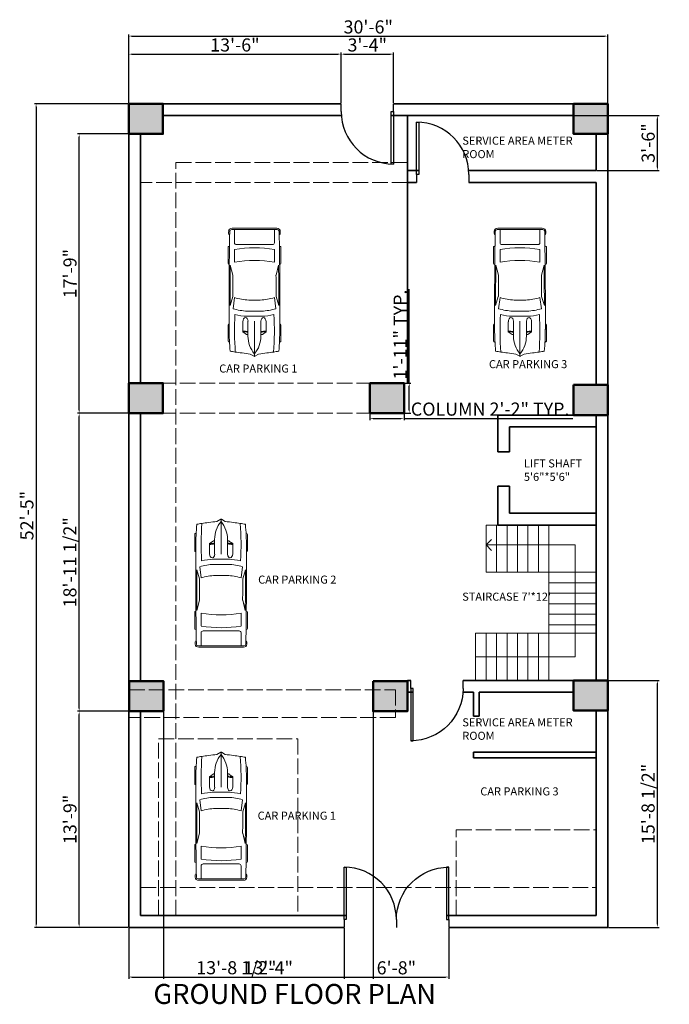
# Model space of a CAD drawing. Units: inches. Extents: x 1964 to 3462, y 1879 to 2909.
# Tile 1 of 4: x 1964 to 2460, y 2008 to 2759. Entities that reach past the tile are written whole.
import ezdxf

# ---------------------------------------------------------------- set-up
doc = ezdxf.new("R2010")
doc.units = ezdxf.units.IN
doc.linetypes.add('ACAD_ISO02W100', pattern=[15, 12, -3])
for name, color, linetype, lineweight in [('A-ANNO-DIMS', 2, 'Continuous', 18), ('A-ANNO-TEXT', 7, 'Continuous', 35), ('A-AREA-IDEN', 7, 'Continuous', 18), ('A-COLS', 1, 'Continuous', 50), ('A-COLS-PATT', 252, 'Continuous', 13), ('A-DOOR', 4, 'Continuous', 25), ('A-EQPM-VEHI', 8, 'Continuous', 13), ('A-FLOR-EVTR', 7, 'Continuous', 35), ('A-FLOR-OVHD', 8, 'ACAD_ISO02W100', 18), ('A-FLOR-PARK', 8, 'ACAD_ISO02W100', 18), ('A-FLOR-STRS', 3, 'Continuous', 18), ('A-WALL', 7, 'Continuous', 35)]:
    doc.layers.add(name, color=color, linetype=linetype, lineweight=lineweight)
doc.styles.get("Standard").update_dxf_attribs({"font": 'arial.ttf'})
doc.dimstyles.new('ISO-25', dxfattribs={"dimtxt": 10, "dimasz": 2.5, "dimexe": 1.25, "dimexo": 0.625, "dimtad": 1, "dimdec": 0, "dimlunit": 4, "dimtxsty": 'Standard', "dimcen": 2.5, "dimadec": 0, "dimazin": 0, "dimtfac": 1, "dimtdec": 0, "dimtmove": 0, "dimatfit": 3, "dimfxl": 1, "dimarcsym": 0})

# ---------------------------------------------------------------- blocks, each defined once
blk = doc.blocks.new('*U2')
for p, q in [((0, 0), (0, -6)), ((40, 0), (40, -6))]:
    blk.add_line(p, q)
blk.add_lwpolyline([(0, 0), (0, 40), (1.75, 40), (1.75, 0)], close=True)
blk.add_arc((0, 0), 40, 0, 90)
blk = doc.blocks.new('*U5')
for p, q in [((21.1, 37.4), (21.1, 36.8)), ((46.6, 38.9), (22.4, 38.9)), ((47.8, 37.4), (47.8, 37.4)), ((70, 31.5), (86.4, 29.4)), ((88, 31.9), (74.8, 35.9)), ((134.3, 35.6), (119.3, 31.8)), ((135.5, 37.1), (135.5, 37.4)), ((136.7, 38.9), (160.9, 38.9)), ((138.4, 29.4), (157.2, 29.4)), ((162.1, 37.4), (162.1, 36.8)), ((186.5, 29.4), (167, 29.4)), ((186.5, -33.5), (186.5, 33.5)), ((188.4, -32.8), (188.4, 32.8)), ((32.3, 11.6), (36.1, 17.2)), ((36.1, 17.2), (50.9, 17.2)), ((164.5, 26.4), (164.5, -26.4)), ((3.3, 6.1), (0.1, 0.4)), ((29.8, 9.5), (51.7, 9.5)), ((32.1, 9.5), (32.1, 11.2)), ((58.9, -10.8), (58.9, 10.8)), ((66.6, -10.5), (66.6, 10.5)), ((82.7, 8.5), (82.7, -8.5)), ((186.5, -10.5), (186.5, 10.5)), ((0, 0), (51.7, 0)), ((0.1, -0.4), (3.3, -6.1)), ((29.8, -9.5), (51.7, -9.5)), ((32.1, -9.5), (32.1, -11.2)), ((32.3, -11.6), (36.1, -17.2)), ((36.1, -17.2), (50.9, -17.2)), ((21.1, -37.4), (21.1, -36.8)), ((46.6, -38.9), (22.4, -38.9)), ((47.8, -37.4), (47.8, -37.4)), ((86.4, -29.4), (70, -31.5)), ((88, -31.9), (74.8, -35.9)), ((134.3, -35.6), (119.3, -31.8)), ((135.5, -37.1), (135.5, -37.4)), ((136.7, -38.9), (160.9, -38.9)), ((157.2, -29.4), (138.4, -29.4)), ((162.1, -37.4), (162.1, -36.8)), ((167, -29.4), (186.5, -29.4))]:
    blk.add_line(p, q)
for centre, major_axis, ratio, start_param, end_param in [((266, -27.5), (0, 313.3), 0.842304, 1.367076, 1.39176), ((37.5, -594), (0, -623.3), 0.842304, 3.096046, 3.200911), ((41.2, -490.9), (0, 528.2), 0.842304, 0.00281, 0.075598), ((22.4, 37.4), (0, -1.48), 0.842304, 3.141593, 4.712389), ((64.5, -10555.6), (0, 10593), 0.842304, -0.013397, 0.002797), ((46.6, 37.4), (0, 1.48), 0.842304, -1.570796, 0), ((135.3, 5.4), (0, 81.8), 0.842304, 1.245306, 1.50788), ((64.5, -10555.6), (0, -10591.5), 0.842304, 3.133765, 3.140441), ((149.6, 2.8), (0, -79.6), 0.842304, 4.372215, 4.640744), ((95.8, -3666.4), (0, -3698.2), 0.842304, 3.134049, 3.144098), ((136.7, 37.4), (0, -1.48), 0.842304, 3.141593, 4.712389), ((17.1, 0), (0, 147), 0.842304, 4.511394, 4.913384), ((35.9, 0), (0, 147), 0.842304, 4.511394, 4.913384), ((160.9, 37.4), (0, 1.48), 0.842304, -1.570796, 0), ((167, 26.4), (0, 2.96), 0.842304, 0, 1.570796), ((180.6, 35.8), (0, 2.22), 0.842304, -0.013017, 1.249894), ((64.5, -10556.4), (0, 10595.3), 0.842304, -0.013397, -0.013017), ((184, 32.8), (0, -5.25), 0.842304, 1.570796, 3.128196), ((184, 33.5), (0, -2.96), 0.842304, 1.570796, 3.128196), ((-204.5, 52.4), (0, -251), 0.842304, 1.385369, 1.434372), ((259.2, -27.5), (0, -305.3), 0.842304, 4.528606, 4.561838), ((13, 17), (0, 27.4), 0.842304, 4.435146, 4.718221), ((14.2, 17), (0, 27.4), 0.842304, 4.435146, 4.718221), ((50.8, 13.3), (6.34, -0.36), 0.603834, -1.395552, 1.581315), ((134.4, 5.4), (0, -89.8), 0.842304, 4.449482, 4.652344), ((0.6, 0), (0, -0.74), 0.842304, 4.131459, 5.293319), ((29.8, -46.7), (0, 56.2), 0.842304, 0, 0.590319), ((32.7, 11.2), (0, 0.74), 0.842304, 0.879714, 1.570796), ((-204.5, -52.4), (0, 251), 0.842304, -1.434372, -1.385369), ((29.8, 46.7), (0, 56.2), 0.842304, 2.551274, 3.141593), ((32.7, -11.2), (0, -0.74), 0.842304, 4.712389, 5.403472), ((13, -17), (0, -27.4), 0.842304, 1.564964, 1.848039), ((14.2, -17), (0, -27.4), 0.842304, 1.564964, 1.848039), ((134.4, -5.4), (0, -89.8), 0.842304, -1.510751, -1.307889), ((135.3, -5.4), (0, -81.8), 0.842304, -1.50788, -1.245306), ((149.6, -2.8), (0, -79.6), 0.842304, -1.499151, -1.230623), ((259.2, 27.5), (0, 305.3), 0.842304, 1.721348, 1.754579), ((266, 27.5), (0, 313.3), 0.842304, 1.749832, 1.774517), ((37.5, 594), (0, -623.3), 0.842304, -0.059319, 0.045547), ((167, -26.4), (0, -2.96), 0.842304, 4.712389, 6.283185), ((41.2, 490.9), (0, -528.2), 0.842304, -0.075598, -0.00281), ((22.4, -37.4), (0, 1.48), 0.842304, 1.570796, 3.141593), ((64.5, 10555.6), (0, 10593), 0.842304, 3.138796, 3.15499), ((46.6, -37.4), (0, -1.48), 0.842304, 0, 1.570796), ((64.5, 10555.6), (0, -10591.5), 0.842304, 0.001152, 0.007828), ((95.8, 3666.4), (0, -3698.2), 0.842304, -0.002505, 0.007544), ((136.7, -37.4), (0, -1.48), 0.842304, -1.570796, 0), ((160.9, -37.4), (0, 1.48), 0.842304, 3.141593, 4.712389), ((180.6, -35.8), (0, -2.22), 0.842304, -1.249894, 0.013017), ((64.5, 10556.4), (0, 10595.3), 0.842304, 3.15461, 3.15499), ((184, -32.8), (0, -5.25), 0.842304, 0.013397, 1.570796), ((184, -33.5), (0, 2.96), 0.842304, 3.15499, 4.712389)]:
    blk.add_ellipse(centre, major_axis=major_axis, ratio=ratio, start_param=start_param, end_param=end_param)
at = {"extrusion": (0, 0, -1)}
blk.add_ellipse((50.8, -13.3), major_axis=(6.34, 0.36), ratio=0.603834, start_param=-1.395552, end_param=1.581315, dxfattribs=at)
blk = doc.blocks.new('*D7')
at = {"layer": 'A-ANNO-DIMS', "color": 0, "lineweight": -2, "transparency": 16777216}
for p, q in [((2047.23, 2695.8), (2047.23, 2748.04)), ((2049.73, 2746.79), (2410.73, 2746.79)), ((2413.23, 2695.8), (2413.23, 2748.04))]:
    blk.add_line(p, q, dxfattribs=at)
at = {"layer": 'A-ANNO-DIMS', "color": 0, "lineweight": 100, "transparency": 16777216}
for points in [[(2049.73, 2747.21), (2049.73, 2746.37), (2047.23, 2746.79)], [(2410.73, 2747.21), (2410.73, 2746.37), (2413.23, 2746.79)]]:
    blk.add_solid(points, dxfattribs=at)
at = {"layer": 'Defpoints', "color": 0, "lineweight": 100, "transparency": 16777216}
for p in [(2413.23, 2746.79), (2047.23, 2695.18), (2413.23, 2695.18)]:
    blk.add_point(p, dxfattribs=at)
at = {"layer": 'A-ANNO-DIMS', "color": 0, "transparency": 16777216, "insert": (2230.23, 2752.52), "char_height": 10, "attachment_point": 5}
blk.add_mtext('30\'-6"', dxfattribs=at)
blk = doc.blocks.new('*D8')
at = {"layer": 'A-ANNO-DIMS', "color": 0, "lineweight": -2, "transparency": 16777216}
for p, q in [((2046.6, 2695.18), (1975.23, 2695.18)), ((1976.48, 2692.68), (1976.48, 2068.92)), ((2046.6, 2066.42), (1975.23, 2066.42))]:
    blk.add_line(p, q, dxfattribs=at)
at = {"layer": 'A-ANNO-DIMS', "color": 0, "lineweight": 100, "transparency": 16777216}
for points in [[(1976.07, 2692.68), (1976.9, 2692.68), (1976.48, 2695.18)], [(1976.07, 2068.92), (1976.9, 2068.92), (1976.48, 2066.42)]]:
    blk.add_solid(points, dxfattribs=at)
at = {"layer": 'Defpoints', "color": 0, "lineweight": 100, "transparency": 16777216}
for p in [(2047.23, 2695.18), (1976.48, 2066.42), (2047.23, 2066.42)]:
    blk.add_point(p, dxfattribs=at)
at = {"layer": 'A-ANNO-DIMS', "color": 0, "transparency": 16777216, "insert": (1970.75, 2380.8), "char_height": 10, "attachment_point": 5, "rotation": 90}
blk.add_mtext('52\'-5"', dxfattribs=at)
blk = doc.blocks.new('COL-RECT-26x23')
blk.add_lwpolyline([(0, 23.08), (26.15, 23.08), (26.15, 0), (0, 0)], close=True)
blk = doc.blocks.new('*D23')
at = {"layer": 'A-ANNO-DIMS', "color": 0, "lineweight": -2, "transparency": 16777216}
for p, q in [((2231.42, 2458.3), (2231.42, 2453.75)), ((2257.57, 2458.3), (2257.57, 2453.75)), ((2233.92, 2455), (2255.07, 2455)), ((2257.57, 2455), (2386.58, 2455))]:
    blk.add_line(p, q, dxfattribs=at)
at = {"layer": 'A-ANNO-DIMS', "color": 0, "lineweight": 100, "transparency": 16777216}
for points in [[(2233.92, 2455.42), (2233.92, 2454.59), (2231.42, 2455)], [(2255.07, 2455.42), (2255.07, 2454.59), (2257.57, 2455)]]:
    blk.add_solid(points, dxfattribs=at)
at = {"layer": 'Defpoints', "color": 0, "lineweight": 100, "transparency": 16777216}
for p in [(2231.42, 2458.93), (2257.57, 2458.93), (2257.57, 2455)]:
    blk.add_point(p, dxfattribs=at)
at = {"layer": 'A-ANNO-DIMS', "color": 0, "transparency": 16777216, "insert": (2323.32, 2460.8), "char_height": 10, "attachment_point": 5}
blk.add_mtext('COLUMN 2\'-2" TYP.', dxfattribs=at)
blk = doc.blocks.new('*D24')
at = {"layer": 'A-ANNO-DIMS', "color": 0, "lineweight": -2, "transparency": 16777216}
for p, q in [((2261.49, 2482.01), (2261.49, 2553.54)), ((2258.19, 2482.01), (2262.74, 2482.01)), ((2261.49, 2461.43), (2261.49, 2479.51)), ((2258.19, 2458.93), (2262.74, 2458.93))]:
    blk.add_line(p, q, dxfattribs=at)
at = {"layer": 'A-ANNO-DIMS', "color": 0, "lineweight": 100, "transparency": 16777216}
for points in [[(2261.08, 2479.51), (2261.91, 2479.51), (2261.49, 2482.01)], [(2261.08, 2461.43), (2261.91, 2461.43), (2261.49, 2458.93)]]:
    blk.add_solid(points, dxfattribs=at)
at = {"layer": 'Defpoints', "color": 0, "lineweight": 100, "transparency": 16777216}
for p in [(2257.57, 2482.01), (2261.49, 2482.01), (2257.57, 2458.93)]:
    blk.add_point(p, dxfattribs=at)
at = {"layer": 'A-ANNO-DIMS', "color": 0, "transparency": 16777216, "insert": (2255.84, 2519.03), "char_height": 10, "attachment_point": 5, "rotation": 90}
blk.add_mtext('1\'-11" TYP.', dxfattribs=at)
blk = doc.blocks.new('*D43')
at = {"layer": 'A-ANNO-DIMS', "color": 0, "lineweight": -2, "transparency": 16777216}
for p, q in [((2047.23, 2065.79), (2047.23, 2027.32)), ((2211.69, 2065.79), (2211.69, 2027.32)), ((2049.73, 2028.57), (2209.19, 2028.57))]:
    blk.add_line(p, q, dxfattribs=at)
at = {"layer": 'A-ANNO-DIMS', "color": 0, "lineweight": 100, "transparency": 16777216}
for points in [[(2049.73, 2028.98), (2049.73, 2028.15), (2047.23, 2028.57)], [(2209.19, 2028.98), (2209.19, 2028.15), (2211.69, 2028.57)]]:
    blk.add_solid(points, dxfattribs=at)
at = {"layer": 'Defpoints', "color": 0, "lineweight": 100, "transparency": 16777216}
for p in [(2047.23, 2066.42), (2211.69, 2066.42), (2211.69, 2028.57)]:
    blk.add_point(p, dxfattribs=at)
at = {"layer": 'A-ANNO-DIMS', "color": 0, "transparency": 16777216, "insert": (2129.46, 2034.37), "char_height": 10, "attachment_point": 5}
blk.add_mtext('13\'-8 1/2"', dxfattribs=at)
blk = doc.blocks.new('*D44')
at = {"layer": 'A-ANNO-DIMS', "color": 0, "lineweight": -2, "transparency": 16777216}
for p, q in [((2211.69, 2065.79), (2211.69, 2027.32)), ((2291.69, 2065.79), (2291.69, 2027.32)), ((2214.19, 2028.57), (2289.19, 2028.57))]:
    blk.add_line(p, q, dxfattribs=at)
at = {"layer": 'A-ANNO-DIMS', "color": 0, "lineweight": 100, "transparency": 16777216}
for points in [[(2214.19, 2028.98), (2214.19, 2028.15), (2211.69, 2028.57)], [(2289.19, 2028.98), (2289.19, 2028.15), (2291.69, 2028.57)]]:
    blk.add_solid(points, dxfattribs=at)
at = {"layer": 'Defpoints', "color": 0, "lineweight": 100, "transparency": 16777216}
for p in [(2211.69, 2066.42), (2291.69, 2066.42), (2291.69, 2028.57)]:
    blk.add_point(p, dxfattribs=at)
at = {"layer": 'A-ANNO-DIMS', "color": 0, "transparency": 16777216, "insert": (2251.69, 2034.3), "char_height": 10, "attachment_point": 5}
blk.add_mtext('6\'-8"', dxfattribs=at)
blk = doc.blocks.new('*D45')
at = {"layer": 'A-ANNO-DIMS', "color": 0, "lineweight": -2, "transparency": 16777216}
for p, q in [((2046.96, 2231.42), (2008.13, 2231.42)), ((2009.38, 2068.92), (2009.38, 2228.92)), ((2046.6, 2066.42), (2008.13, 2066.42))]:
    blk.add_line(p, q, dxfattribs=at)
at = {"layer": 'A-ANNO-DIMS', "color": 0, "lineweight": 100, "transparency": 16777216}
for points in [[(2008.96, 2228.92), (2009.8, 2228.92), (2009.38, 2231.42)], [(2008.96, 2068.92), (2009.8, 2068.92), (2009.38, 2066.42)]]:
    blk.add_solid(points, dxfattribs=at)
at = {"layer": 'Defpoints', "color": 0, "lineweight": 100, "transparency": 16777216}
for p in [(2009.38, 2231.42), (2047.58, 2231.42), (2047.23, 2066.42)]:
    blk.add_point(p, dxfattribs=at)
at = {"layer": 'A-ANNO-DIMS', "color": 0, "transparency": 16777216, "insert": (2003.64, 2148.92), "char_height": 10, "attachment_point": 5, "rotation": 90}
blk.add_mtext('13\'-9"', dxfattribs=at)
blk = doc.blocks.new('*D46')
at = {"layer": 'A-ANNO-DIMS', "color": 0, "lineweight": -2, "transparency": 16777216}
for p, q in [((2046.6, 2458.93), (2008.13, 2458.93)), ((2009.38, 2233.92), (2009.38, 2456.43)), ((2046.96, 2231.42), (2008.13, 2231.42))]:
    blk.add_line(p, q, dxfattribs=at)
at = {"layer": 'A-ANNO-DIMS', "color": 0, "lineweight": 100, "transparency": 16777216}
for points in [[(2008.96, 2456.43), (2009.8, 2456.43), (2009.38, 2458.93)], [(2008.96, 2233.92), (2009.8, 2233.92), (2009.38, 2231.42)]]:
    blk.add_solid(points, dxfattribs=at)
at = {"layer": 'Defpoints', "color": 0, "lineweight": 100, "transparency": 16777216}
for p in [(2009.38, 2458.93), (2047.23, 2458.93), (2047.58, 2231.42)]:
    blk.add_point(p, dxfattribs=at)
at = {"layer": 'A-ANNO-DIMS', "color": 0, "transparency": 16777216, "insert": (2003.58, 2345.17), "char_height": 10, "attachment_point": 5, "rotation": 90}
blk.add_mtext('18\'-11 1/2"', dxfattribs=at)
blk = doc.blocks.new('*D47')
at = {"layer": 'A-ANNO-DIMS', "color": 0, "lineweight": -2, "transparency": 16777216}
for p, q in [((2046.6, 2672.1), (2008.13, 2672.1)), ((2009.38, 2461.43), (2009.38, 2669.6)), ((2046.6, 2458.93), (2008.13, 2458.93))]:
    blk.add_line(p, q, dxfattribs=at)
at = {"layer": 'A-ANNO-DIMS', "color": 0, "lineweight": 100, "transparency": 16777216}
for points in [[(2008.96, 2669.6), (2009.8, 2669.6), (2009.38, 2672.1)], [(2008.96, 2461.43), (2009.8, 2461.43), (2009.38, 2458.93)]]:
    blk.add_solid(points, dxfattribs=at)
at = {"layer": 'Defpoints', "color": 0, "lineweight": 100, "transparency": 16777216}
for p in [(2009.38, 2672.1), (2047.23, 2672.1), (2047.23, 2458.93)]:
    blk.add_point(p, dxfattribs=at)
at = {"layer": 'A-ANNO-DIMS', "color": 0, "transparency": 16777216, "insert": (2003.65, 2565.51), "char_height": 10, "attachment_point": 5, "rotation": 90}
blk.add_mtext('17\'-9"', dxfattribs=at)
blk = doc.blocks.new('*D48')
at = {"layer": 'A-ANNO-DIMS', "color": 0, "lineweight": -2, "transparency": 16777216}
for p, q in [((2047.23, 2695.8), (2047.23, 2734.28)), ((2049.73, 2733.03), (2206.97, 2733.03)), ((2209.47, 2695.8), (2209.47, 2734.28))]:
    blk.add_line(p, q, dxfattribs=at)
at = {"layer": 'A-ANNO-DIMS', "color": 0, "lineweight": 100, "transparency": 16777216}
for points in [[(2049.73, 2733.45), (2049.73, 2732.61), (2047.23, 2733.03)], [(2206.97, 2733.45), (2206.97, 2732.61), (2209.47, 2733.03)]]:
    blk.add_solid(points, dxfattribs=at)
at = {"layer": 'Defpoints', "color": 0, "lineweight": 100, "transparency": 16777216}
for p in [(2209.47, 2733.03), (2047.23, 2695.18), (2209.47, 2695.18)]:
    blk.add_point(p, dxfattribs=at)
at = {"layer": 'A-ANNO-DIMS', "color": 0, "transparency": 16777216, "insert": (2128.35, 2738.76), "char_height": 10, "attachment_point": 5}
blk.add_mtext('13\'-6"', dxfattribs=at)
blk = doc.blocks.new('*D49')
at = {"layer": 'A-ANNO-DIMS', "color": 0, "lineweight": -2, "transparency": 16777216}
for p, q in [((2209.47, 2695.8), (2209.47, 2734.28)), ((2211.97, 2733.03), (2246.97, 2733.03)), ((2249.47, 2695.8), (2249.47, 2734.28))]:
    blk.add_line(p, q, dxfattribs=at)
at = {"layer": 'A-ANNO-DIMS', "color": 0, "lineweight": 100, "transparency": 16777216}
for points in [[(2211.97, 2733.45), (2211.97, 2732.61), (2209.47, 2733.03)], [(2246.97, 2733.45), (2246.97, 2732.61), (2249.47, 2733.03)]]:
    blk.add_solid(points, dxfattribs=at)
at = {"layer": 'Defpoints', "color": 0, "lineweight": 100, "transparency": 16777216}
for p in [(2249.47, 2733.03), (2209.47, 2695.18), (2249.47, 2695.18)]:
    blk.add_point(p, dxfattribs=at)
at = {"layer": 'A-ANNO-DIMS', "color": 0, "transparency": 16777216, "insert": (2229.47, 2738.76), "char_height": 10, "attachment_point": 5}
blk.add_mtext('3\'-4"', dxfattribs=at)
blk = doc.blocks.new('*D50')
at = {"layer": 'A-ANNO-DIMS', "color": 0, "lineweight": -2, "transparency": 16777216}
for p, q in [((2413.85, 2255.01), (2452.33, 2255.01)), ((2451.08, 2068.92), (2451.08, 2252.51)), ((2413.85, 2066.42), (2452.33, 2066.42))]:
    blk.add_line(p, q, dxfattribs=at)
at = {"layer": 'A-ANNO-DIMS', "color": 0, "lineweight": 100, "transparency": 16777216}
for points in [[(2450.66, 2252.51), (2451.5, 2252.51), (2451.08, 2255.01)], [(2450.66, 2068.92), (2451.5, 2068.92), (2451.08, 2066.42)]]:
    blk.add_solid(points, dxfattribs=at)
at = {"layer": 'Defpoints', "color": 0, "lineweight": 100, "transparency": 16777216}
for p in [(2413.23, 2255.01), (2451.08, 2255.01), (2413.23, 2066.42)]:
    blk.add_point(p, dxfattribs=at)
at = {"layer": 'A-ANNO-DIMS', "color": 0, "transparency": 16777216, "insert": (2445.28, 2160.71), "char_height": 10, "attachment_point": 5, "rotation": 90}
blk.add_mtext('15\'-8 1/2"', dxfattribs=at)
blk = doc.blocks.new('*D51')
at = {"layer": 'A-ANNO-DIMS', "color": 0, "lineweight": -2, "transparency": 16777216}
for p, q in [((2073.74, 2230.79), (2073.74, 2027.32)), ((2233.96, 2230.79), (2233.96, 2027.32)), ((2076.24, 2028.57), (2231.46, 2028.57))]:
    blk.add_line(p, q, dxfattribs=at)
at = {"layer": 'A-ANNO-DIMS', "color": 0, "lineweight": 100, "transparency": 16777216}
for points in [[(2076.24, 2028.98), (2076.24, 2028.15), (2073.74, 2028.57)], [(2231.46, 2028.98), (2231.46, 2028.15), (2233.96, 2028.57)]]:
    blk.add_solid(points, dxfattribs=at)
at = {"layer": 'Defpoints', "color": 0, "lineweight": 100, "transparency": 16777216}
for p in [(2073.74, 2231.42), (2233.96, 2231.42), (2233.96, 2028.57)]:
    blk.add_point(p, dxfattribs=at)
at = {"layer": 'A-ANNO-DIMS', "color": 0, "transparency": 16777216, "insert": (2153.85, 2034.3), "char_height": 10, "attachment_point": 5}
blk.add_mtext('13\'-4"', dxfattribs=at)
blk = doc.blocks.new('*D52')
at = {"layer": 'A-ANNO-DIMS', "color": 0, "lineweight": -2, "transparency": 16777216}
for p, q in [((2387.7, 2686.18), (2452.33, 2686.18)), ((2451.08, 2646.68), (2451.08, 2683.68)), ((2404.85, 2644.18), (2452.33, 2644.18))]:
    blk.add_line(p, q, dxfattribs=at)
at = {"layer": 'A-ANNO-DIMS', "color": 0, "lineweight": 100, "transparency": 16777216}
for points in [[(2450.66, 2683.68), (2451.5, 2683.68), (2451.08, 2686.18)], [(2450.66, 2646.68), (2451.5, 2646.68), (2451.08, 2644.18)]]:
    blk.add_solid(points, dxfattribs=at)
at = {"layer": 'Defpoints', "color": 0, "lineweight": 100, "transparency": 16777216}
for p in [(2387.07, 2686.18), (2451.08, 2686.18), (2404.23, 2644.18)]:
    blk.add_point(p, dxfattribs=at)
at = {"layer": 'A-ANNO-DIMS', "color": 0, "transparency": 16777216, "insert": (2445.34, 2665.18), "char_height": 10, "attachment_point": 5, "rotation": 90}
blk.add_mtext('3\'-6"', dxfattribs=at)

msp = doc.modelspace()

# ---------------------------------------------------------------- hatches: boundary and pattern name
at = {"layer": 'A-COLS-PATT'}
h = msp.add_hatch(color=256, dxfattribs=at)
h.dxf.hatch_style = 1
h.paths.add_polyline_path([(2073.38, 2695.18), (2047.23, 2695.18), (2047.23, 2672.1), (2073.38, 2672.1)])
h.paths.add_polyline_path([(2413.23, 2695.18), (2387.07, 2695.18), (2387.07, 2672.1), (2413.23, 2672.1)])
h.paths.add_polyline_path([(2413.23, 2480.62), (2387.07, 2480.62), (2387.07, 2457.54), (2404.23, 2457.54), (2413.23, 2457.54)])
h.paths.add_polyline_path([(2257.57, 2482.01), (2231.42, 2482.01), (2231.42, 2458.93), (2257.57, 2458.93)])
h.paths.add_polyline_path([(2073.38, 2482.01), (2056.23, 2482.01), (2047.23, 2482.01), (2047.23, 2458.93), (2073.38, 2458.93)])
h.paths.add_polyline_path([(2073.74, 2247.83), (2047.58, 2247.83), (2047.58, 2231.42), (2073.74, 2231.42)])
h.paths.add_polyline_path([(2073.74, 2254.5), (2047.58, 2254.5), (2047.58, 2247.83), (2073.74, 2247.83)])
h.paths.add_polyline_path([(2251.13, 2247.83), (2233.96, 2247.83), (2233.96, 2231.42), (2251.13, 2231.42)], flags=17)
h.paths.add_polyline_path([(2260.11, 2254.5), (2233.96, 2254.5), (2233.96, 2247.83), (2251.13, 2247.83), (2251.13, 2231.42), (2260.11, 2231.42)])
h.paths.add_polyline_path([(2413.23, 2255.01), (2404.23, 2255.01), (2404.23, 2254.93), (2387.07, 2254.93), (2387.07, 2231.93), (2413.23, 2231.93)])

# ---------------------------------------------------------------- linework, layer by layer
at = {"layer": 'A-FLOR-EVTR'}
for p, q in [((2329.23, 2457.54), (2329.23, 2429.38)), ((2404.23, 2457.54), (2329.23, 2457.54)), ((2404.23, 2448.54), (2338.23, 2448.54)), ((2338.23, 2448.54), (2338.23, 2429.38)), ((2329.23, 2429.38), (2338.23, 2429.38)), ((2329.23, 2403.23), (2338.23, 2403.23)), ((2329.23, 2403.23), (2329.23, 2373.54)), ((2338.23, 2403.23), (2338.23, 2382.54)), ((2338.23, 2382.54), (2404.23, 2382.54)), ((2329.23, 2373.54), (2404.23, 2373.54))]:
    msp.add_line(p, q, dxfattribs=at)
at = {"layer": 'A-FLOR-OVHD'}
for p, q in [((2056.23, 2482.01), (2260.23, 2482.01)), ((2056.23, 2458.93), (2257.57, 2458.93))]:
    msp.add_line(p, q, dxfattribs=at)
msp.add_lwpolyline([(2047.58, 2247.83), (2251.13, 2247.83), (2251.13, 2226.58), (2047.58, 2226.58)], close=True, dxfattribs=at)
at = {"layer": 'A-FLOR-PARK'}
for p, q in [((2083.21, 2075.42), (2083.21, 2650.24)), ((2083.21, 2650.24), (2260.23, 2650.24)), ((2260.23, 2635.18), (2056.23, 2635.18)), ((2297.34, 2075.42), (2297.34, 2141.01)), ((2297.34, 2141.01), (2404.23, 2141.01)), ((2056.23, 2096.92), (2404.23, 2096.92))]:
    msp.add_line(p, q, dxfattribs=at)
msp.add_lwpolyline([(2176.39, 2075.42), (2070.07, 2075.42), (2070.07, 2210.48), (2176.39, 2210.48)], close=True, dxfattribs=at)
at = {"layer": 'A-FLOR-STRS'}
for p, q in [((2320.23, 2337.54), (2320.23, 2373.54)), ((2320.23, 2373.54), (2346.76, 2373.54)), ((2328.23, 2337.54), (2328.23, 2373.54)), ((2336.23, 2337.54), (2336.23, 2373.54)), ((2344.23, 2337.54), (2344.23, 2373.54)), ((2352.23, 2337.54), (2352.23, 2373.54)), ((2360.23, 2337.54), (2360.23, 2373.54)), ((2368.23, 2337.54), (2368.23, 2373.54)), ((2404.23, 2373.54), (2404.23, 2337.54)), ((2320.23, 2358.41), (2324.46, 2362.55)), ((2388.17, 2358.41), (2320.23, 2358.41)), ((2320.23, 2358.41), (2324.46, 2354.28)), ((2388.17, 2272.93), (2388.17, 2358.41)), ((2368.23, 2337.54), (2320.23, 2337.54)), ((2368.23, 2290.93), (2368.23, 2337.54)), ((2368.23, 2337.54), (2404.23, 2337.54)), ((2368.23, 2329.54), (2404.23, 2329.54)), ((2368.23, 2321.54), (2404.23, 2321.54)), ((2368.23, 2313.54), (2404.23, 2313.54)), ((2368.23, 2305.54), (2404.23, 2305.54)), ((2368.23, 2297.54), (2404.23, 2297.54)), ((2312.23, 2290.93), (2312.23, 2254.93)), ((2335.61, 2290.93), (2312.23, 2290.93)), ((2320.23, 2290.93), (2320.23, 2254.93)), ((2328.23, 2290.93), (2328.23, 2254.93)), ((2368.23, 2290.93), (2335.61, 2290.93)), ((2336.23, 2290.93), (2336.23, 2254.93)), ((2344.23, 2290.93), (2344.23, 2254.93)), ((2352.23, 2290.93), (2352.23, 2254.93)), ((2360.23, 2290.93), (2360.23, 2254.93)), ((2368.23, 2290.93), (2404.23, 2290.93)), ((2368.23, 2290.93), (2368.23, 2254.93)), ((2404.23, 2254.93), (2404.23, 2290.93)), ((2312.23, 2272.93), (2388.17, 2272.93)), ((2404.23, 2254.93), (2368.23, 2254.93))]:
    msp.add_line(p, q, dxfattribs=at)
at = {"layer": 'A-WALL'}
for p, q in [((2073.38, 2686.17), (2209.59, 2686.05)), ((2260.23, 2684.62), (2260.23, 2686.18)), ((2260.23, 2686.01), (2260.23, 2482.01)), ((2404.23, 2672.1), (2404.23, 2644.18)), ((2268.77, 2644.18), (2260.23, 2644.18)), ((2404.23, 2644.18), (2306.9, 2644.18)), ((2267.02, 2635.18), (2260.23, 2635.18)), ((2404.23, 2635.18), (2307.02, 2635.18)), ((2056.23, 2458.93), (2056.23, 2254.93)), ((2056.23, 2458.93), (2056.23, 2254.93)), ((2260.23, 2254.93), (2260.23, 2245.93)), ((2262.66, 2254.93), (2260.23, 2254.93)), ((2320.23, 2254.93), (2302.66, 2254.93)), ((2404.23, 2254.93), (2320.23, 2254.93)), ((2260.23, 2245.93), (2264.41, 2245.93)), ((2302.55, 2245.93), (2310.49, 2245.93)), ((2310.49, 2245.93), (2310.49, 2227.8)), ((2314.99, 2245.93), (2314.99, 2227.8)), ((2314.99, 2245.93), (2387.07, 2245.93)), ((2047.23, 2231.42), (2047.23, 2066.42)), ((2056.23, 2231.42), (2056.23, 2075.42)), ((2310.49, 2227.8), (2314.99, 2227.8)), ((2314.99, 2200.29), (2310.49, 2200.29)), ((2310.49, 2200.29), (2310.49, 2195.79)), ((2404.23, 2195.79), (2310.49, 2195.79)), ((2404.23, 2200.29), (2314.99, 2200.29)), ((2404.23, 2075.42), (2404.23, 2179.29)), ((2413.23, 2066.42), (2413.23, 2179.29)), ((2056.23, 2075.42), (2213.44, 2075.42)), ((2251.58, 2075.42), (2251.81, 2075.42)), ((2289.94, 2075.42), (2404.23, 2075.42)), ((2047.23, 2066.42), (2211.69, 2066.42)), ((2291.69, 2066.42), (2413.23, 2066.42))]:
    msp.add_line(p, q, dxfattribs=at)
for points in [[(2209.47, 2695.18), (2047.23, 2695.18), (2047.23, 2156.26)], [(2413.23, 2156.26), (2413.23, 2695.18), (2249.47, 2695.18)], [(2209.58, 2686.18), (2073.38, 2686.18)], [(2387.07, 2686.18), (2247.72, 2686.18)], [(2056.23, 2672.1), (2056.23, 2482.01)], [(2404.23, 2644.18), (2404.23, 2672.1)], [(2404.23, 2480.62), (2404.23, 2635.18)], [(2056.23, 2458.93), (2056.23, 2254.5)], [(2404.23, 2254.93), (2404.23, 2457.54)], [(2056.23, 2231.42), (2056.23, 2165.26)], [(2404.23, 2165.26), (2404.23, 2231.93)]]:
    msp.add_lwpolyline(points, dxfattribs=at)

# ---------------------------------------------------------------- block references
at = {"layer": 'A-COLS'}
for p in [(2047.23, 2672.1), (2387.07, 2672.1), (2047.23, 2458.93), (2231.42, 2458.93), (2387.07, 2457.54), (2387.07, 2231.93), (2047.58, 2231.42), (2233.96, 2231.42)]:
    msp.add_blockref('COL-RECT-26x23', p, dxfattribs=at)
at = {"layer": 'A-DOOR', "rotation": 180}
msp.add_blockref('*U2', (2249.47, 2689.18), dxfattribs=at)
at = {"layer": 'A-DOOR'}
for p in [(2267.02, 2641.18), (2211.69, 2072.42)]:
    msp.add_blockref('*U2', p, dxfattribs=at)
at = {"layer": 'A-DOOR', "xscale": -1, "rotation": 180}
msp.add_blockref('*U2', (2262.66, 2248.93), dxfattribs=at)
at = {"layer": 'A-DOOR', "xscale": -1}
msp.add_blockref('*U2', (2291.69, 2072.42), dxfattribs=at)
at = {"layer": 'A-EQPM-VEHI', "xscale": 0.5189507813375265, "yscale": 0.5189507813375265, "zscale": 0.5189507813375265}
for p, rotation in [((2143.28, 2502.35), 89.99999999999999), ((2346.11, 2502.35), 89.99999999999999), ((2117.81, 2378.11), 270), ((2117.81, 2200.24), 270)]:
    msp.add_blockref('*U5', p, dxfattribs=dict(at, rotation=rotation))

# ---------------------------------------------------------------- texts
at = {"layer": 'A-ANNO-TEXT', "insert": (2066.08, 2023.28), "char_height": 15.2607, "attachment_point": 1}
msp.add_mtext_dynamic_manual_height_columns('GROUND FLOOR PLAN', width=480.7827, gutter_width=76.3, heights=[0], dxfattribs=at)
at = {"layer": 'A-AREA-IDEN', "attachment_point": 1}
for s, insert, char_height in [('SERVICE AREA METER\\PROOM', (2302.09, 2670.07), 6.1611), ('CAR PARKING 1', (2116.39, 2496.14), 6.1611), ('CAR PARKING 3', (2322.43, 2499.49), 6.1611), ('LIFT SHAFT\\P5\'6"*5\'6"', (2349.11, 2423.73), 6.161), ('CAR PARKING 2', (2146.11, 2335.01), 6.1611), ("STAIRCASE 7'*12'", (2301.98, 2321.99), 6.1611), ('SERVICE AREA METER\\PROOM', (2302.09, 2226.07), 6.1611), ('CAR PARKING 3', (2315.82, 2173.36), 6.1611), ('CAR PARKING 1', (2145.73, 2154.83), 6.1611)]:
    msp.add_mtext_dynamic_manual_height_columns(s, width=194.1034, gutter_width=30.81, heights=[0], dxfattribs=dict(at, insert=insert, char_height=char_height))

# ---------------------------------------------------------------- dimensions: what is measured, and where the dimension line sits
at = {"layer": 'A-ANNO-DIMS'}
for base, p1, p2, override, picture, middle in [((2413.23, 2746.79), (2047.23, 2695.18), (2413.23, 2695.18), {"dimclrd": 0, "dimclre": 0, "dimclrt": 0}, '*D7', (2230.23, 2752.52)), ((2209.47, 2733.03), (2047.23, 2695.18), (2209.47, 2695.18), {"dimdec": 1, "dimlfac": 1, "dimrnd": 0, "dimzin": 1, "dimdsep": 46, "dimlunit": 4, "dimfrac": 2}, '*D48', (2128.35, 2738.76)), ((2249.47, 2733.03), (2209.47, 2695.18), (2249.47, 2695.18), {"dimdec": 1, "dimlfac": 1, "dimrnd": 0, "dimzin": 1, "dimdsep": 46, "dimlunit": 4, "dimfrac": 2}, '*D49', (2229.47, 2738.76)), ((2233.96, 2028.57), (2073.74, 2231.42), (2233.96, 2231.42), {"dimdec": 1, "dimlfac": 1, "dimrnd": 0, "dimzin": 1, "dimdsep": 46, "dimlunit": 4, "dimfrac": 2}, '*D51', (2153.85, 2034.3)), ((2211.69, 2028.57), (2047.23, 2066.42), (2211.69, 2066.42), {"dimdec": 1, "dimlfac": 1, "dimrnd": 0, "dimzin": 1, "dimdsep": 46, "dimlunit": 4, "dimfrac": 2}, '*D43', (2129.46, 2034.37)), ((2291.69, 2028.57), (2211.69, 2066.42), (2291.69, 2066.42), {"dimdec": 1, "dimlfac": 1, "dimrnd": 0, "dimzin": 1, "dimdsep": 46, "dimlunit": 4, "dimfrac": 2}, '*D44', (2251.69, 2034.3))]:
    dim = msp.add_linear_dim(base=base, p1=p1, p2=p2, dimstyle='ISO-25', override=override, dxfattribs=at)
    dim.commit()
    dim.dimension.update_dxf_attribs({"geometry": picture, "text_midpoint": middle})
for base, p1, p2, override, picture, middle in [((1976.48, 2066.42), (2047.23, 2695.18), (2047.23, 2066.42), {"dimclrd": 0, "dimclre": 0, "dimclrt": 0}, '*D8', (1970.75, 2380.8)), ((2451.08, 2686.18), (2404.23, 2644.18), (2387.07, 2686.18), {"dimdec": 1, "dimlfac": 1, "dimrnd": 0, "dimzin": 1, "dimdsep": 46, "dimlunit": 4, "dimfrac": 2}, '*D52', (2445.34, 2665.18)), ((2009.38, 2672.1), (2047.23, 2458.93), (2047.23, 2672.1), {"dimdec": 1, "dimlfac": 1, "dimrnd": 0, "dimzin": 1, "dimdsep": 46, "dimlunit": 4, "dimfrac": 2}, '*D47', (2003.65, 2565.51)), ((2009.38, 2458.93), (2047.58, 2231.42), (2047.23, 2458.93), {"dimdec": 1, "dimlfac": 1, "dimrnd": 0, "dimzin": 1, "dimdsep": 46, "dimlunit": 4, "dimfrac": 2}, '*D46', (2003.58, 2345.17)), ((2451.08, 2255.01), (2413.23, 2066.42), (2413.23, 2255.01), {"dimdec": 1, "dimlfac": 1, "dimrnd": 0, "dimzin": 1, "dimdsep": 46, "dimlunit": 4, "dimfrac": 2}, '*D50', (2445.28, 2160.71)), ((2009.38, 2231.42), (2047.23, 2066.42), (2047.58, 2231.42), {"dimdec": 1, "dimlfac": 1, "dimrnd": 0, "dimzin": 1, "dimdsep": 46, "dimlunit": 4, "dimfrac": 2}, '*D45', (2003.64, 2148.92))]:
    dim = msp.add_linear_dim(base=base, p1=p1, p2=p2, angle=90, dimstyle='ISO-25', override=override, dxfattribs=at)
    dim.commit()
    dim.dimension.update_dxf_attribs({"geometry": picture, "text_midpoint": middle})
dim = msp.add_linear_dim(base=(2261.49, 2482.01), p1=(2257.57, 2458.93), p2=(2257.57, 2482.01), angle=90, text='<> TYP.', dimstyle='ISO-25', override={"dimdec": 1, "dimlfac": 1, "dimrnd": 0, "dimzin": 1, "dimdsep": 46, "dimlunit": 4, "dimfrac": 2}, dxfattribs=at)
dim.commit()
dim.dimension.update_dxf_attribs({"geometry": '*D24', "text_midpoint": (2255.84, 2519.03)})
dim = msp.add_linear_dim(base=(2257.5699, 2455.003), p1=(2231.4153, 2458.9262), p2=(2257.5699, 2458.9262), text='COLUMN <> TYP.', dimstyle='ISO-25', override={"dimdec": 1, "dimlfac": 1, "dimrnd": 0, "dimzin": 1, "dimdsep": 46, "dimlunit": 4, "dimfrac": 2}, dxfattribs=at)
dim.commit()
dim.dimension.update_dxf_attribs({"geometry": '*D23', "text_midpoint": (2323.3245, 2460.802)})

doc.saveas('drawing.dxf')
